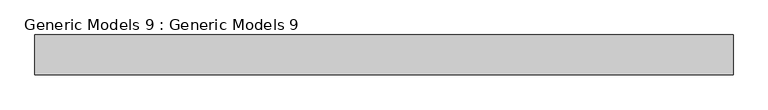
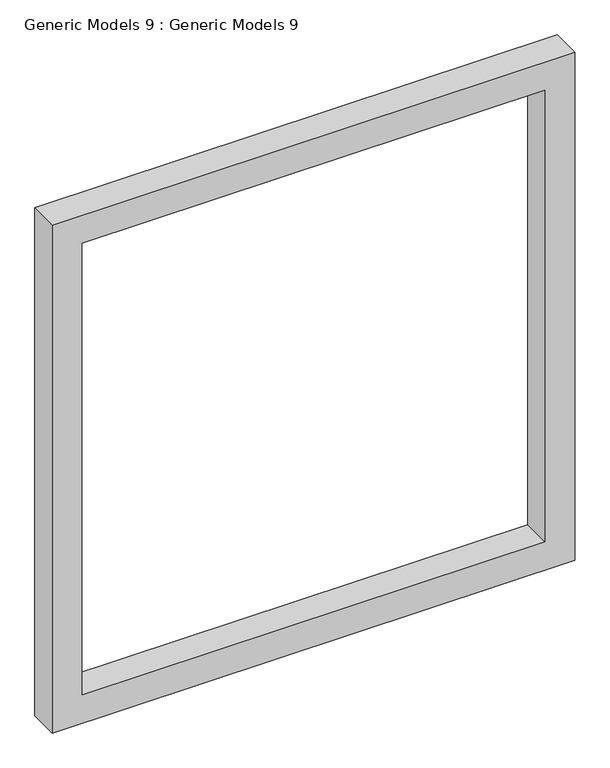
"""IFC4 building model written with IfcOpenShell, lengths in millimetres: proxy geometry, Generic Models 9 : Generic Models 9."""

from ifc_helpers import new_model, si_unit, frame, origin, place, context, project, spatial, polyline, outline, extrude, source, transform, mapped, element, save


def generic_models_9_generic_models_9_ba76ca7f(model_context):
    return source(origin(), model_context, "Body", "SweptSolid", [
        extrude(outline(polyline([(2673.5634674, -7405.8495061), (845.8670086, -7405.8495061), (845.8670086, -5627.8495061), (2673.5634674, -5627.8495061), (2673.5634674, -7405.8495061)]), holes=[polyline([(2571.9634674, -7304.2495061), (2571.9634674, -5729.4495061), (947.4670086, -5729.4495061), (947.4670086, -7304.2495061), (2571.9634674, -7304.2495061)])]), frame((0.0, -10372.9896616, 0.0), z_axis=(0.0, 1.0, 0.0), x_axis=(0.0, 0.0, 1.0)), (0.0, 0.0, 1.0), 101.6),
    ])


if __name__ == "__main__":
    model = new_model("IFC4")
    model_context = context("Model", 3, world=origin())
    ifc_project = project(units=[si_unit("LENGTHUNIT", "METRE", prefix="MILLI")], contexts=[model_context])
    site = spatial("IfcSite", under=ifc_project)
    building = spatial("IfcBuilding", under=site)
    placement = place(None, origin())
    generic_models_9_generic_models_9_shape = generic_models_9_generic_models_9_ba76ca7f(model_context)
    element("IfcBuildingElementProxy", 1, Name="Generic Models 9 : Generic Models 9", ObjectType="Generic Models 9 : Generic Models 9", at=placement, inside=building, context=model_context, shape_type="MappedRepresentation", body=[
        mapped(generic_models_9_generic_models_9_shape, transform((0.0, 0.0, 0.0), x_axis=(1.0, 0.0, 0.0), y_axis=(0.0, 1.0, 0.0), z_axis=(0.0, 0.0, 1.0))),
    ])
    save(model, "model.ifc")

# Revit data of these elements
# Element 1 (IfcBuildingElementProxy, "Generic Models 9 : Generic Models 9")
#   Materials on its faces: "ACCENT BEIGE COLOUR"
# Materials
#   "ACCENT BEIGE COLOUR": class "Generic", colour RGB 120 120 120, transparency 0, Cost = 0
